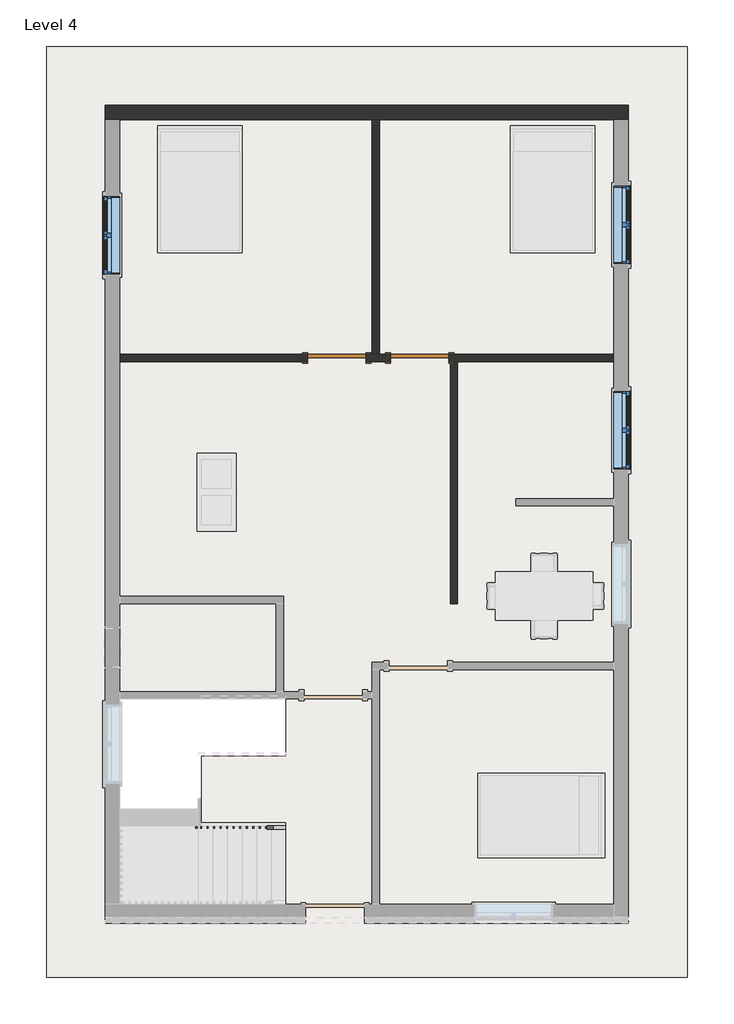
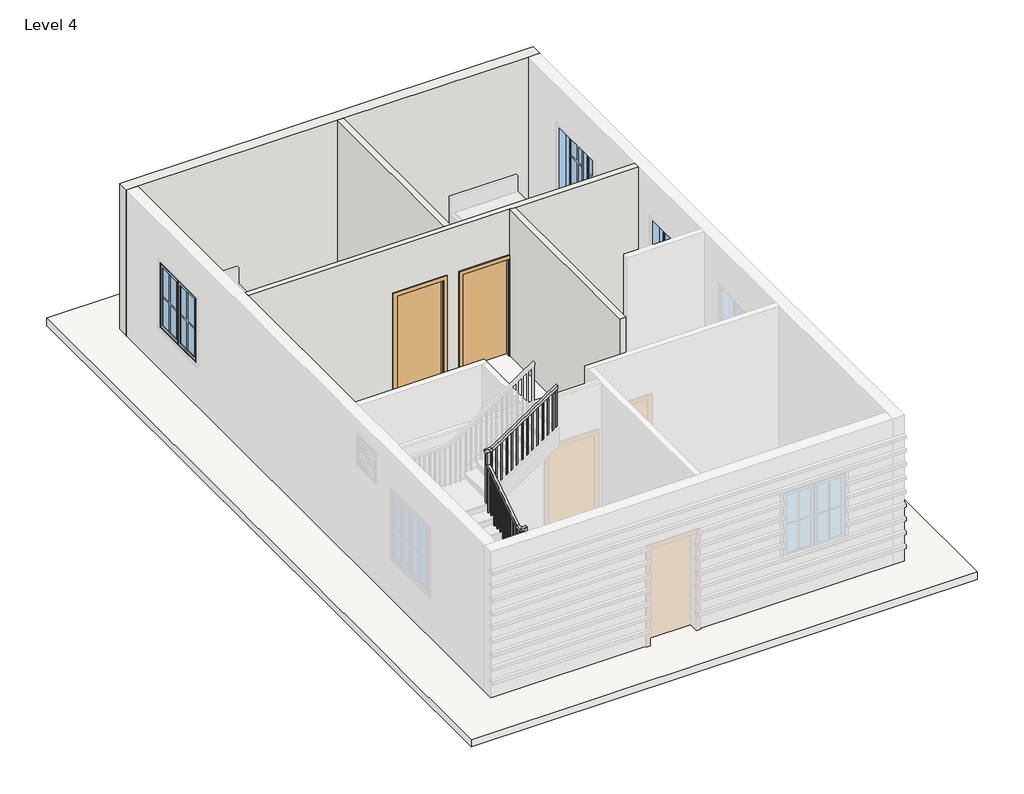
# One storey, part 2 of 3: 4 walls, 3 windows, 2 doors, 1 railing, 1 roof.
"""IFC4 building model written with IfcOpenShell, lengths in millimetres."""

from ifc_helpers import new_model, si_unit, frame, origin, place, context, project, spatial, polyline, outline, extrude, faceted_brep, transform, mapped, element, save
from components import single_flush_door_3_17d80c48, single_flush_door_3_5e62189b, window_casement_double_window_4_576b2d2c

model = new_model("IFC4")

# Units and contexts
model_context = context("Model", 3, world=origin())
ifc_project = project(units=[si_unit("LENGTHUNIT", "METRE", prefix="MILLI")], contexts=[model_context])

# Site, building, storey
site = spatial("IfcSite", under=ifc_project)
building = spatial("IfcBuilding", under=site)
storey = spatial("IfcBuildingStorey", under=building, Name="Level 4", Elevation=9448.8)

# Doors
placement = place(None, origin())
single_flush_door_3_shape = single_flush_door_3_17d80c48(model_context)
element("IfcDoor", 1, ObjectType="Single-Flush : DOOR 3'", at=placement, inside=storey, context=model_context, shape_type="MappedRepresentation", body=[
    mapped(single_flush_door_3_shape, transform((-1721.4617403, 2133.1073441, 9448.8), x_axis=(1.0, 0.0, 0.0), y_axis=(0.0, 1.0, 0.0), z_axis=(0.0, 0.0, 1.0))),
])
single_flush_door_3_2_shape = single_flush_door_3_5e62189b(model_context)
element("IfcDoor", 2, ObjectType="Single-Flush : DOOR 3'", at=placement, inside=storey, context=model_context, shape_type="MappedRepresentation", body=[
    mapped(single_flush_door_3_2_shape, transform((-426.0617403, 2133.1073441, 9448.8), x_axis=(-1.0, 0.0, 0.0), y_axis=(0.0, -1.0, 0.0), z_axis=(0.0, 0.0, 1.0))),
])

# Railing
element("IfcRailing", 3, ObjectType="Handrail - Rectangular", at=placement, inside=storey, context=model_context, shape_type="SolidModel", body=[
    faceted_brep([(-2515.2117403, -5213.8426559, 10515.6), (-2515.2117403, -5213.8426559, 10454.5459984), (-2515.2117403, -5163.0426559, 10454.5459984), (-2515.2117403, -5163.0426559, 10515.6), (-3810.6117403, -5213.8426559, 11379.2), (-3861.4117403, -5213.8426559, 11352.0126651), (-3861.4117403, -5163.0426559, 11352.0126651), (-3810.6117403, -5163.0426559, 11379.2), (-3810.6117403, -5213.8426559, 11633.2), (-3861.4117403, -5213.8426559, 11582.4), (-3861.4117403, -5163.0426559, 11582.4), (-3810.6117403, -5163.0426559, 11633.2), (-3937.6117403, -5213.8426559, 11633.2), (-3937.6117403, -5213.8426559, 11582.4), (-3886.8117403, -5163.0426559, 11582.4), (-3886.8117403, -5163.0426559, 11633.2), (-3937.6117403, -5086.8426559, 11633.2), (-3937.6117403, -5071.4616535, 11582.4), (-3886.8117403, -5071.4616535, 11582.4), (-3886.8117403, -5086.8426559, 11633.2), (-3937.6117403, -4096.2426559, 12293.6), (-3937.6117403, -4045.4426559, 12266.4126651), (-3886.8117403, -4045.4426559, 12266.4126651), (-3886.8117403, -4096.2426559, 12293.6), (-3937.6117403, -4096.2426559, 12547.6), (-3937.6117403, -4045.4426559, 12496.8), (-3886.8117403, -4045.4426559, 12496.8), (-3886.8117403, -4096.2426559, 12547.6), (-3937.6117403, -3969.2426559, 12547.6), (-3937.6117403, -3969.2426559, 12496.8), (-3886.8117403, -4020.0426559, 12496.8), (-3886.8117403, -4020.0426559, 12547.6), (-3810.6117403, -3969.2426559, 12547.6), (-3795.2307379, -3969.2426559, 12496.8), (-3795.2307379, -4020.0426559, 12496.8), (-3810.6117403, -4020.0426559, 12547.6), (-2515.2117403, -3969.2426559, 13411.2), (-2515.2117403, -4020.0426559, 13411.2), (-2515.2117403, -4020.0426559, 13350.1459984), (-2515.2117403, -3969.2426559, 13350.1459984)], [[[0, 1, 2, 3]], [[1, 0, 4, 5]], [[2, 1, 5, 6]], [[3, 2, 6, 7]], [[0, 3, 7, 4]], [[5, 4, 8, 9]], [[6, 5, 9, 10]], [[7, 6, 10, 11]], [[4, 7, 11, 8]], [[9, 8, 12, 13]], [[10, 9, 13, 14]], [[11, 10, 14, 15]], [[8, 11, 15, 12]], [[13, 12, 16, 17]], [[14, 13, 17, 18]], [[15, 14, 18, 19]], [[12, 15, 19, 16]], [[17, 16, 20, 21]], [[18, 17, 21, 22]], [[19, 18, 22, 23]], [[16, 19, 23, 20]], [[21, 20, 24, 25]], [[22, 21, 25, 26]], [[23, 22, 26, 27]], [[20, 23, 27, 24]], [[25, 24, 28, 29]], [[26, 25, 29, 30]], [[27, 26, 30, 31]], [[24, 27, 31, 28]], [[29, 28, 32, 33]], [[30, 29, 33, 34]], [[31, 30, 34, 35]], [[28, 31, 35, 32]], [[36, 37, 38, 39]], [[33, 32, 36, 39]], [[34, 33, 39, 38]], [[35, 34, 38, 37]], [[32, 35, 37, 36]]]),
    extrude(outline(polyline([(13305.6959984, -2581.8867403), (13292.9959984, -2600.9367403), (12344.4, -2600.9367403), (12344.4, -2581.8867403), (13305.6959984, -2581.8867403)])), frame((0.0, -4004.1676559, 0.0), z_axis=(0.0, 1.0, 0.0), x_axis=(0.0, 0.0, 1.0)), (0.0, 0.0, 1.0), 19.05),
    extrude(outline(polyline([(13237.9626651, -2683.4867403), (13225.2626651, -2702.5367403), (12344.4, -2702.5367403), (12344.4, -2683.4867403), (13237.9626651, -2683.4867403)])), frame((0.0, -4004.1676559, 0.0), z_axis=(0.0, 1.0, 0.0), x_axis=(0.0, 0.0, 1.0)), (0.0, 0.0, 1.0), 19.05),
    extrude(outline(polyline([(13170.2293317, -2785.0867403), (13157.5293317, -2804.1367403), (12192.0, -2804.1367403), (12192.0, -2785.0867403), (13170.2293317, -2785.0867403)])), frame((0.0, -4004.1676559, 0.0), z_axis=(0.0, 1.0, 0.0), x_axis=(0.0, 0.0, 1.0)), (0.0, 0.0, 1.0), 19.05),
    extrude(outline(polyline([(13102.4959984, -2886.6867403), (13089.7959984, -2905.7367403), (12192.0, -2905.7367403), (12192.0, -2886.6867403), (13102.4959984, -2886.6867403)])), frame((0.0, -4004.1676559, 0.0), z_axis=(0.0, 1.0, 0.0), x_axis=(0.0, 0.0, 1.0)), (0.0, 0.0, 1.0), 19.05),
    extrude(outline(polyline([(13034.7626651, -2988.2867403), (13022.0626651, -3007.3367403), (12039.6, -3007.3367403), (12039.6, -2988.2867403), (13034.7626651, -2988.2867403)])), frame((0.0, -4004.1676559, 0.0), z_axis=(0.0, 1.0, 0.0), x_axis=(0.0, 0.0, 1.0)), (0.0, 0.0, 1.0), 19.05),
    extrude(outline(polyline([(12967.0293317, -3089.8867403), (12954.3293317, -3108.9367403), (12039.6, -3108.9367403), (12039.6, -3089.8867403), (12967.0293317, -3089.8867403)])), frame((0.0, -4004.1676559, 0.0), z_axis=(0.0, 1.0, 0.0), x_axis=(0.0, 0.0, 1.0)), (0.0, 0.0, 1.0), 19.05),
    extrude(outline(polyline([(12899.2959984, -3191.4867403), (12886.5959984, -3210.5367403), (12039.6, -3210.5367403), (12039.6, -3191.4867403), (12899.2959984, -3191.4867403)])), frame((0.0, -4004.1676559, 0.0), z_axis=(0.0, 1.0, 0.0), x_axis=(0.0, 0.0, 1.0)), (0.0, 0.0, 1.0), 19.05),
    extrude(outline(polyline([(12831.5626651, -3293.0867403), (12818.8626651, -3312.1367403), (11887.2, -3312.1367403), (11887.2, -3293.0867403), (12831.5626651, -3293.0867403)])), frame((0.0, -4004.1676559, 0.0), z_axis=(0.0, 1.0, 0.0), x_axis=(0.0, 0.0, 1.0)), (0.0, 0.0, 1.0), 19.05),
    extrude(outline(polyline([(12763.8293317, -3394.6867403), (12751.1293317, -3413.7367403), (11887.2, -3413.7367403), (11887.2, -3394.6867403), (12763.8293317, -3394.6867403)])), frame((0.0, -4004.1676559, 0.0), z_axis=(0.0, 1.0, 0.0), x_axis=(0.0, 0.0, 1.0)), (0.0, 0.0, 1.0), 19.05),
    extrude(outline(polyline([(12696.0959984, -3496.2867403), (12683.3959984, -3515.3367403), (11734.8, -3515.3367403), (11734.8, -3496.2867403), (12696.0959984, -3496.2867403)])), frame((0.0, -4004.1676559, 0.0), z_axis=(0.0, 1.0, 0.0), x_axis=(0.0, 0.0, 1.0)), (0.0, 0.0, 1.0), 19.05),
    extrude(outline(polyline([(12628.3626651, -3597.8867403), (12615.6626651, -3616.9367403), (11734.8, -3616.9367403), (11734.8, -3597.8867403), (12628.3626651, -3597.8867403)])), frame((0.0, -4004.1676559, 0.0), z_axis=(0.0, 1.0, 0.0), x_axis=(0.0, 0.0, 1.0)), (0.0, 0.0, 1.0), 19.05),
    extrude(outline(polyline([(12560.6293317, -3699.4867403), (12547.9293317, -3718.5367403), (11582.4, -3718.5367403), (11582.4, -3699.4867403), (12560.6293317, -3699.4867403)])), frame((0.0, -4004.1676559, 0.0), z_axis=(0.0, 1.0, 0.0), x_axis=(0.0, 0.0, 1.0)), (0.0, 0.0, 1.0), 19.05),
    extrude(outline(polyline([(12492.8959984, -3801.0867403), (12480.1959984, -3820.1367403), (11582.4, -3820.1367403), (11582.4, -3801.0867403), (12492.8959984, -3801.0867403)])), frame((0.0, -4004.1676559, 0.0), z_axis=(0.0, 1.0, 0.0), x_axis=(0.0, 0.0, 1.0)), (0.0, 0.0, 1.0), 19.05),
    extrude(outline(polyline([(-3902.6867403, -4080.3676559), (-3921.7367403, -4080.3676559), (-3921.7367403, -4061.3176559), (-3902.6867403, -4061.3176559), (-3902.6867403, -4080.3676559)])), frame((0.0, 0.0, 11277.6), z_axis=(0.0, 0.0, 1.0), x_axis=(1.0, 0.0, 0.0)), (0.0, 0.0, 1.0), 1219.2),
    extrude(outline(polyline([(-4181.9676559, 12175.3959984), (-4162.9176559, 12188.0959984), (-4162.9176559, 11277.6), (-4181.9676559, 11277.6), (-4181.9676559, 12175.3959984)])), frame((-3921.7367403, 0.0, 0.0), z_axis=(1.0, 0.0, 0.0), x_axis=(0.0, 1.0, 0.0)), (0.0, 0.0, 1.0), 19.05),
    extrude(outline(polyline([(-4283.5676559, 12107.6626651), (-4264.5176559, 12120.3626651), (-4264.5176559, 11125.2), (-4283.5676559, 11125.2), (-4283.5676559, 12107.6626651)])), frame((-3921.7367403, 0.0, 0.0), z_axis=(1.0, 0.0, 0.0), x_axis=(0.0, 1.0, 0.0)), (0.0, 0.0, 1.0), 19.05),
    extrude(outline(polyline([(-4385.1676559, 12039.9293317), (-4366.1176559, 12052.6293317), (-4366.1176559, 11125.2), (-4385.1676559, 11125.2), (-4385.1676559, 12039.9293317)])), frame((-3921.7367403, 0.0, 0.0), z_axis=(1.0, 0.0, 0.0), x_axis=(0.0, 1.0, 0.0)), (0.0, 0.0, 1.0), 19.05),
    extrude(outline(polyline([(-4486.7676559, 11972.1959984), (-4467.7176559, 11984.8959984), (-4467.7176559, 11125.2), (-4486.7676559, 11125.2), (-4486.7676559, 11972.1959984)])), frame((-3921.7367403, 0.0, 0.0), z_axis=(1.0, 0.0, 0.0), x_axis=(0.0, 1.0, 0.0)), (0.0, 0.0, 1.0), 19.05),
    extrude(outline(polyline([(-4588.3676559, 11904.4626651), (-4569.3176559, 11917.1626651), (-4569.3176559, 10972.8), (-4588.3676559, 10972.8), (-4588.3676559, 11904.4626651)])), frame((-3921.7367403, 0.0, 0.0), z_axis=(1.0, 0.0, 0.0), x_axis=(0.0, 1.0, 0.0)), (0.0, 0.0, 1.0), 19.05),
    extrude(outline(polyline([(-4689.9676559, 11836.7293317), (-4670.9176559, 11849.4293317), (-4670.9176559, 10972.8), (-4689.9676559, 10972.8), (-4689.9676559, 11836.7293317)])), frame((-3921.7367403, 0.0, 0.0), z_axis=(1.0, 0.0, 0.0), x_axis=(0.0, 1.0, 0.0)), (0.0, 0.0, 1.0), 19.05),
    extrude(outline(polyline([(-4791.5676559, 11768.9959984), (-4772.5176559, 11781.6959984), (-4772.5176559, 10820.4), (-4791.5676559, 10820.4), (-4791.5676559, 11768.9959984)])), frame((-3921.7367403, 0.0, 0.0), z_axis=(1.0, 0.0, 0.0), x_axis=(0.0, 1.0, 0.0)), (0.0, 0.0, 1.0), 19.05),
    extrude(outline(polyline([(-4893.1676559, 11701.2626651), (-4874.1176559, 11713.9626651), (-4874.1176559, 10820.4), (-4893.1676559, 10820.4), (-4893.1676559, 11701.2626651)])), frame((-3921.7367403, 0.0, 0.0), z_axis=(1.0, 0.0, 0.0), x_axis=(0.0, 1.0, 0.0)), (0.0, 0.0, 1.0), 19.05),
    extrude(outline(polyline([(-4994.7676559, 11633.5293317), (-4975.7176559, 11646.2293317), (-4975.7176559, 10668.0), (-4994.7676559, 10668.0), (-4994.7676559, 11633.5293317)])), frame((-3921.7367403, 0.0, 0.0), z_axis=(1.0, 0.0, 0.0), x_axis=(0.0, 1.0, 0.0)), (0.0, 0.0, 1.0), 19.05),
    extrude(outline(polyline([(-5096.3676559, 11565.7959984), (-5077.3176559, 11578.4959984), (-5077.3176559, 10668.0), (-5096.3676559, 10668.0), (-5096.3676559, 11565.7959984)])), frame((-3921.7367403, 0.0, 0.0), z_axis=(1.0, 0.0, 0.0), x_axis=(0.0, 1.0, 0.0)), (0.0, 0.0, 1.0), 19.05),
    extrude(outline(polyline([(-3826.4867403, -5178.9176559), (-3826.4867403, -5197.9676559), (-3845.5367403, -5197.9676559), (-3845.5367403, -5178.9176559), (-3826.4867403, -5178.9176559)])), frame((0.0, 0.0, 10363.2), z_axis=(0.0, 0.0, 1.0), x_axis=(1.0, 0.0, 0.0)), (0.0, 0.0, 1.0), 1219.2),
    extrude(outline(polyline([(11260.9959984, -3724.8867403), (11273.6959984, -3743.9367403), (10363.2, -3743.9367403), (10363.2, -3724.8867403), (11260.9959984, -3724.8867403)])), frame((0.0, -5197.9676559, 0.0), z_axis=(0.0, 1.0, 0.0), x_axis=(0.0, 0.0, 1.0)), (0.0, 0.0, 1.0), 19.05),
    extrude(outline(polyline([(11193.2626651, -3623.2867403), (11205.9626651, -3642.3367403), (10210.8, -3642.3367403), (10210.8, -3623.2867403), (11193.2626651, -3623.2867403)])), frame((0.0, -5197.9676559, 0.0), z_axis=(0.0, 1.0, 0.0), x_axis=(0.0, 0.0, 1.0)), (0.0, 0.0, 1.0), 19.05),
    extrude(outline(polyline([(11125.5293317, -3521.6867403), (11138.2293317, -3540.7367403), (10210.8, -3540.7367403), (10210.8, -3521.6867403), (11125.5293317, -3521.6867403)])), frame((0.0, -5197.9676559, 0.0), z_axis=(0.0, 1.0, 0.0), x_axis=(0.0, 0.0, 1.0)), (0.0, 0.0, 1.0), 19.05),
    extrude(outline(polyline([(11057.7959984, -3420.0867403), (11070.4959984, -3439.1367403), (10210.8, -3439.1367403), (10210.8, -3420.0867403), (11057.7959984, -3420.0867403)])), frame((0.0, -5197.9676559, 0.0), z_axis=(0.0, 1.0, 0.0), x_axis=(0.0, 0.0, 1.0)), (0.0, 0.0, 1.0), 19.05),
    extrude(outline(polyline([(10990.0626651, -3318.4867403), (11002.7626651, -3337.5367403), (10058.4, -3337.5367403), (10058.4, -3318.4867403), (10990.0626651, -3318.4867403)])), frame((0.0, -5197.9676559, 0.0), z_axis=(0.0, 1.0, 0.0), x_axis=(0.0, 0.0, 1.0)), (0.0, 0.0, 1.0), 19.05),
    extrude(outline(polyline([(10922.3293317, -3216.8867403), (10935.0293317, -3235.9367403), (10058.4, -3235.9367403), (10058.4, -3216.8867403), (10922.3293317, -3216.8867403)])), frame((0.0, -5197.9676559, 0.0), z_axis=(0.0, 1.0, 0.0), x_axis=(0.0, 0.0, 1.0)), (0.0, 0.0, 1.0), 19.05),
    extrude(outline(polyline([(10854.5959984, -3115.2867403), (10867.2959984, -3134.3367403), (9906.0, -3134.3367403), (9906.0, -3115.2867403), (10854.5959984, -3115.2867403)])), frame((0.0, -5197.9676559, 0.0), z_axis=(0.0, 1.0, 0.0), x_axis=(0.0, 0.0, 1.0)), (0.0, 0.0, 1.0), 19.05),
    extrude(outline(polyline([(10786.8626651, -3013.6867403), (10799.5626651, -3032.7367403), (9906.0, -3032.7367403), (9906.0, -3013.6867403), (10786.8626651, -3013.6867403)])), frame((0.0, -5197.9676559, 0.0), z_axis=(0.0, 1.0, 0.0), x_axis=(0.0, 0.0, 1.0)), (0.0, 0.0, 1.0), 19.05),
    extrude(outline(polyline([(10719.1293317, -2912.0867403), (10731.8293317, -2931.1367403), (9753.6, -2931.1367403), (9753.6, -2912.0867403), (10719.1293317, -2912.0867403)])), frame((0.0, -5197.9676559, 0.0), z_axis=(0.0, 1.0, 0.0), x_axis=(0.0, 0.0, 1.0)), (0.0, 0.0, 1.0), 19.05),
    extrude(outline(polyline([(10651.3959984, -2810.4867403), (10664.0959984, -2829.5367403), (9753.6, -2829.5367403), (9753.6, -2810.4867403), (10651.3959984, -2810.4867403)])), frame((0.0, -5197.9676559, 0.0), z_axis=(0.0, 1.0, 0.0), x_axis=(0.0, 0.0, 1.0)), (0.0, 0.0, 1.0), 19.05),
    extrude(outline(polyline([(10583.6626651, -2708.8867403), (10596.3626651, -2727.9367403), (9601.2, -2727.9367403), (9601.2, -2708.8867403), (10583.6626651, -2708.8867403)])), frame((0.0, -5197.9676559, 0.0), z_axis=(0.0, 1.0, 0.0), x_axis=(0.0, 0.0, 1.0)), (0.0, 0.0, 1.0), 19.05),
    extrude(outline(polyline([(10515.9293317, -2607.2867403), (10528.6293317, -2626.3367403), (9601.2, -2626.3367403), (9601.2, -2607.2867403), (10515.9293317, -2607.2867403)])), frame((0.0, -5197.9676559, 0.0), z_axis=(0.0, 1.0, 0.0), x_axis=(0.0, 0.0, 1.0)), (0.0, 0.0, 1.0), 19.05),
    extrude(outline(polyline([(-3902.6867403, -4004.1676559), (-3921.7367403, -4004.1676559), (-3921.7367403, -3985.1176559), (-3902.6867403, -3985.1176559), (-3902.6867403, -4004.1676559)])), frame((0.0, 0.0, 11430.0), z_axis=(0.0, 0.0, 1.0), x_axis=(1.0, 0.0, 0.0)), (0.0, 0.0, 1.0), 1066.8),
    extrude(outline(polyline([(-3902.6867403, -5178.9176559), (-3902.6867403, -5197.9676559), (-3921.7367403, -5197.9676559), (-3921.7367403, -5178.9176559), (-3902.6867403, -5178.9176559)])), frame((0.0, 0.0, 10515.6), z_axis=(0.0, 0.0, 1.0), x_axis=(1.0, 0.0, 0.0)), (0.0, 0.0, 1.0), 1066.8),
    extrude(outline(polyline([(13350.1459984, -2515.2117403), (13337.4459984, -2534.2617403), (12344.4, -2534.2617403), (12344.4, -2515.2117403), (13350.1459984, -2515.2117403)])), frame((0.0, -4004.1676559, 0.0), z_axis=(0.0, 1.0, 0.0), x_axis=(0.0, 0.0, 1.0)), (0.0, 0.0, 1.0), 19.05),
    extrude(outline(polyline([(10454.5459984, -2515.2117403), (10467.2459984, -2534.2617403), (9601.2, -2534.2617403), (9601.2, -2515.2117403), (10454.5459984, -2515.2117403)])), frame((0.0, -5197.9676559, 0.0), z_axis=(0.0, 1.0, 0.0), x_axis=(0.0, 0.0, 1.0)), (0.0, 0.0, 1.0), 19.05),
])

# Roof
element("IfcRoof", 4, ObjectType="ROOF 6\"", at=placement, inside=storey, context=model_context, shape_type="SweptSolid", body=[
    extrude(outline(polyline([(-6249.0117403, -7525.2426559), (-6249.0117403, 6990.8573441), (3745.8882597, 6990.8573441), (3745.8882597, -7525.2426559), (-6249.0117403, -7525.2426559)]), holes=[polyline([(-5156.8117403, -3131.0426559), (-5156.8117403, -6433.0426559), (-2515.2117403, -6433.0426559), (-2515.2117403, -5112.2426559), (-3836.0117403, -5112.2426559), (-3836.0117403, -4070.8426559), (-2515.2117403, -4070.8426559), (-2515.2117403, -3131.0426559), (-5156.8117403, -3131.0426559)])]), frame((0.0, 0.0, 9296.4), z_axis=(0.0, 0.0, 1.0), x_axis=(1.0, 0.0, 0.0)), (0.0, 0.0, 1.0), 152.4),
])

# Walls
element("IfcWall", 5, ObjectType="ALL 4.5\"", at=placement, inside=storey, context=model_context, shape_type="Brep", body=[
    faceted_brep([(-1264.2617403, 2075.9573441, 9448.8), (-883.2617403, 2075.9573441, 9448.8), (-883.2617403, 2075.9573441, 11480.8), (31.1382597, 2075.9573441, 11480.8), (31.1382597, 2075.9573441, 9448.8), (50.1882597, 2075.9573441, 9448.8), (164.4882597, 2075.9573441, 9448.8), (2602.8882597, 2075.9573441, 9448.8), (2602.8882597, 2075.9573441, 12496.8), (164.4882597, 2075.9573441, 12496.8), (50.1882597, 2075.9573441, 12496.8), (-5106.0117403, 2075.9573441, 12496.8), (-5106.0117403, 2075.9573441, 9448.8), (-2178.6617403, 2075.9573441, 9448.8), (-2178.6617403, 2075.9573441, 11480.8), (-1264.2617403, 2075.9573441, 11480.8), (-883.2617403, 2190.2573441, 11480.8), (-883.2617403, 2190.2573441, 9448.8), (-1054.7117403, 2190.2573441, 9448.8), (-1169.0117403, 2190.2573441, 9448.8), (-1264.2617403, 2190.2573441, 9448.8), (-1264.2617403, 2190.2573441, 11480.8), (-2178.6617403, 2190.2573441, 11480.8), (-2178.6617403, 2190.2573441, 9448.8), (-5106.0117403, 2190.2573441, 9448.8), (-5106.0117403, 2190.2573441, 12496.8), (-1169.0117403, 2190.2573441, 12496.8), (-1054.7117403, 2190.2573441, 12496.8), (2602.8882597, 2190.2573441, 12496.8), (2602.8882597, 2190.2573441, 9448.8), (31.1382597, 2190.2573441, 9448.8), (31.1382597, 2190.2573441, 11480.8)], [[[0, 1, 2, 3, 4, 5, 6, 7, 8, 9, 10, 11, 12, 13, 14, 15]], [[16, 17, 18, 19, 20, 21, 22, 23, 24, 25, 26, 27, 28, 29, 30, 31]], [[13, 12, 24, 23]], [[30, 29, 7, 6, 5, 4]], [[20, 19, 18, 17, 1, 0]], [[8, 7, 29, 28]], [[12, 11, 25, 24]], [[21, 20, 0, 15]], [[22, 21, 15, 14]], [[23, 22, 14, 13]], [[2, 1, 17, 16]], [[3, 2, 16, 31]], [[4, 3, 31, 30]], [[11, 10, 9, 8, 28, 27, 26, 25]]]),
])
element("IfcWall", 6, ObjectType="ALL 4.5\"", at=placement, inside=storey, context=model_context, shape_type="SweptSolid", body=[
    extrude(outline(polyline([(50.1882597, -1695.9426559), (50.1882597, 2075.9573441), (164.4882597, 2075.9573441), (164.4882597, -1695.9426559), (50.1882597, -1695.9426559)])), frame((0.0, 0.0, 9448.8), z_axis=(0.0, 0.0, 1.0), x_axis=(1.0, 0.0, 0.0)), (0.0, 0.0, 1.0), 3048.0),
])
element("IfcWall", 7, ObjectType="ALL 4.5\"", at=placement, inside=storey, context=model_context, shape_type="SweptSolid", body=[
    extrude(outline(polyline([(-1169.0117403, 2190.2573441), (-1169.0117403, 5847.8573441), (-1054.7117403, 5847.8573441), (-1054.7117403, 2190.2573441), (-1169.0117403, 2190.2573441)])), frame((0.0, 0.0, 9448.8), z_axis=(0.0, 0.0, 1.0), x_axis=(1.0, 0.0, 0.0)), (0.0, 0.0, 1.0), 3048.0),
])
element("IfcWall", 8, ObjectType="WALL 9\"", at=placement, inside=storey, context=model_context, shape_type="Brep", body=[
    faceted_brep([(-5334.6117403, 5847.8573441, 9448.8), (-5106.0117403, 5847.8573441, 9448.8), (-1169.0117403, 5847.8573441, 9448.8), (-1054.7117403, 5847.8573441, 9448.8), (2602.8882597, 5847.8573441, 9448.8), (2831.4882597, 5847.8573441, 9448.8), (2831.4882597, 5847.8573441, 12496.8), (2602.8882597, 5847.8573441, 12496.8), (-1054.7117403, 5847.8573441, 12496.8), (-1169.0117403, 5847.8573441, 12496.8), (-5106.0117403, 5847.8573441, 12496.8), (-5334.6117403, 5847.8573441, 12496.8), (-5334.6117403, 6076.4573441, 9448.8), (-5334.6117403, 6076.4573441, 12496.8), (2831.4882597, 6076.4573441, 12496.8), (2831.4882597, 6076.4573441, 9448.8)], [[[0, 1, 2, 3, 4, 5, 6, 7, 8, 9, 10, 11]], [[12, 13, 14, 15]], [[5, 4, 3, 2, 1, 0, 12, 15]], [[6, 5, 15, 14]], [[0, 11, 13, 12]], [[11, 10, 9, 8, 7, 6, 14, 13]]]),
])

# Windows
window_casement_double_window_4_shape = window_casement_double_window_4_576b2d2c(model_context)
element("IfcWindow", 9, ObjectType="Window-Casement-Double : WINDOW 4'", at=placement, inside=storey, context=model_context, shape_type="MappedRepresentation", body=[
    mapped(window_casement_double_window_4_shape, transform((-5220.3117403, 4047.6323441, 9448.8), x_axis=(0.0, 1.0, 0.0), y_axis=(-1.0, 0.0, 0.0), z_axis=(0.0, 0.0, 1.0))),
])
element("IfcWindow", 10, ObjectType="Window-Casement-Double : WINDOW 4'", at=placement, inside=storey, context=model_context, shape_type="MappedRepresentation", body=[
    mapped(window_casement_double_window_4_shape, transform((2717.1882597, 4209.5573441, 9448.8), x_axis=(0.0, -1.0, 0.0), y_axis=(1.0, 0.0, 0.0), z_axis=(0.0, 0.0, 1.0))),
])
element("IfcWindow", 11, ObjectType="Window-Casement-Double : WINDOW 4'", at=placement, inside=storey, context=model_context, shape_type="MappedRepresentation", body=[
    mapped(window_casement_double_window_4_shape, transform((2717.1882597, 1009.1573441, 9448.8), x_axis=(0.0, -1.0, 0.0), y_axis=(1.0, 0.0, 0.0), z_axis=(0.0, 0.0, 1.0))),
])

save(model, "model.ifc")

# Revit data of these elements
# Type "Single-Flush : DOOR 3'"
#   Type Mark = "8"
#   Construction Type Id = "MDOOR"
#   Assembly Code = "C1020"
#   Analytic Construction = "Metal"
#   Thickness = 0' - 2"
#   Heat Transfer Coefficient (U) = 0.651978 BTU/(h·ft²·°F)
#   Height = 6' - 8"
#   Trim Projection Ext = 0' - 1"
#   Trim Projection Int = 0' - 1"
#   Trim Width = 0' - 3"
#   Width = 3' - 0"
#   Define Thermal Properties by = 1
#   Door Material = Door - Panel
#   Frame Material = Door - Frame
#   Visual Light Transmittance = 0
#   Solar Heat Gain Coefficient = 0
#   Function = (empty or 0)
#   Wall Closure = (empty or 0)
# Type "Handrail - Rectangular"
#   Assembly Code = "C2010400"
#   built-in parameter 1008612 = 0.0416667 (stored number, unit not read)
#   built-in parameter 1008611 = 0.0416667 (stored number, unit not read)
#   built-in parameter 1008609 = 0.333333 (stored number, unit not read)
#   built-in parameter 1008604 = 0.166667 (stored number, unit not read)
#   built-in parameter 1008603 = 0.166667 (stored number, unit not read)
#   Railing Height = 3' - 0"
#   built-in parameter 1008630 = 2
#   built-in parameter 1008610 = 2
#   built-in parameter 1008618 = Baluster - Square : 3/4"
# Type "ROOF 6\""
#   Assembly Code = "B1020"
#   Layers, outside or top first: 0' - 6" no material (function 1)
# Type "ALL 4.5\""
#   Assembly Code = "B2010"
#   Layers, outside or top first: 0' - 4 1/2" no material (function 1)
# Type "WALL 9\""
#   Assembly Code = "B2010"
#   Layers, outside or top first: 0' - 9" "Carpet (1)" (function 1)
# Type "Window-Casement-Double : WINDOW 4'"
#   Type Mark = "18"
#   Fire Rating = "0.5h"
#   Assembly Code = "B2020100"
#   Analytic Construction = "Double glazing - domestic"
#   Frame Extension [instance default] = 0' - 0 1/4"
#   Window Inset [instance default] = 0' - 0"
#   Wall Thickness [instance default] = 0' - 6"
#   Interior Wall Closure [instance default] = 0' - 2 1/4"
#   Half Width = 2' - 0"
#   Visual Light Transmittance = 0.81
#   Thermal Resistance (R) = 1.8146 (h·ft²·°F)/BTU
#   Solar Heat Gain Coefficient = 0.76
#   Rough Width = 4' - 0 1/2"
#   Rough Height = 4' - 5 1/2"
#   Height = 4' - 5"
#   Heat Transfer Coefficient (U) = 0.5511 BTU/(h·ft²·°F)
#   Exterior Wall Closure [instance default] = 0' - 1 1/4"
#   Extension Jamb [instance default] = 0' - 2 1/4"
#   Default Sill Height = 3' - 0"
#   Width = 4' - 0"
#   Muntin Visibility = yes
#   Interior Trim Visibility [instance default] = yes
#   Exterior Trim Visibility [instance default] = yes
#   Extension Jamb Visibility [instance default] = yes
#   Interior Trim Material = Wood - Stained
#   Muntin Pattern = Muntin Pattern_2x2 : Muntin Pattern_2x2
#   Interior Trim = Trim-Window-Interior-Flat : Picture Frame
#   Interior Frame Material = Wood - Stained
#   Glass Panel Material = Glass
#   Exterior Trim Material = Clad - White
#   Exterior Trim = Trim-Window-Exterior-Flat : with Sill
#   Exterior Frame Material = Clad - White
#   Wall Closure = (empty or 0)
# Elements 1, 2 (IfcDoor, "Single-Flush : DOOR 3'")
#   Phase Created = New Construction
#   Materials on its faces: "Door - Frame", "Door - Panel"
# Element 3 (IfcRailing, "Handrail - Rectangular")
#   Phase Created = New Construction
#   Materials on its faces: "Clad - White"
# Element 4 (IfcRoof, "ROOF 6\"")
#   built-in parameter 1001705 = 31 (stored number, unit not read)
#   built-in parameter 1001701 = -0.5 (stored number, unit not read)
#   built-in parameter 1001710 = 33615
#   Phase Created = New Construction
#   Materials on its faces: "Clad - White", "Default Roof", "Softwood, Lumber"
# Elements 5, 6, 7 (IfcWall, "ALL 4.5\"")
#   Top Offset = 0' - 0"
#   Base Offset = 0' - 0"
#   Unconnected Height = 10' - 0"
#   wall height = 10' - 0"
#   Phase Created = New Construction
#   Base Constraint = Level 4
#   Materials on its faces: "Default Wall"
# Element 8 (IfcWall, "WALL 9\"")
#   Top Offset = 0' - 0"
#   Base Offset = 0' - 0"
#   Unconnected Height = 10' - 0"
#   wall height = 10' - 0"
#   Phase Created = New Construction
#   Base Constraint = Level 4
#   Materials on its faces: "Carpet (1)", "Wood - Stained"
# Element 9 (IfcWindow, "Window-Casement-Double : WINDOW 4'")
#   Mark = "23"
#   Window Inset = 0' - 0"
#   Interior Wall Closure = 0' - 2 1/4"
#   Frame Extension = 0' - 0 1/4"
#   Exterior Wall Closure = 0' - 1 1/4"
#   Interior Trim Visibility = yes
#   Exterior Trim Visibility = yes
#   Phase Created = New Construction
#   Materials on its faces: "Wood - Stained", "Glass", "Clad - White"
# Element 10 (IfcWindow, "Window-Casement-Double : WINDOW 4'")
#   Mark = "24"
#   Window Inset = 0' - 0"
#   Interior Wall Closure = 0' - 2 1/4"
#   Frame Extension = 0' - 0 1/4"
#   Exterior Wall Closure = 0' - 1 1/4"
#   Interior Trim Visibility = yes
#   Exterior Trim Visibility = yes
#   Phase Created = New Construction
#   Materials on its faces: "Wood - Stained", "Glass", "Clad - White"
# Element 11 (IfcWindow, "Window-Casement-Double : WINDOW 4'")
#   Mark = "25"
#   Window Inset = 0' - 0"
#   Interior Wall Closure = 0' - 2 1/4"
#   Frame Extension = 0' - 0 1/4"
#   Exterior Wall Closure = 0' - 1 1/4"
#   Interior Trim Visibility = yes
#   Exterior Trim Visibility = yes
#   Phase Created = New Construction
#   Materials on its faces: "Wood - Stained", "Glass", "Clad - White"
# Materials
#   "Door - Panel": class "Wood", colour RGB 210 159 95, transparency 0, Cost = 0
#   "Door - Frame": colour RGB 118 70 51, transparency 0, Cost = 0
#   "Carpet (1)": class "Carpet", colour RGB 124 80 67, transparency 0, Description = "Interior finish", Cost = 0
#   "Wood - Stained": class "Wood", colour RGB 224 178 126, transparency 0, Cost = 0
#   "Glass": class "Glass", colour RGB 0 128 192, transparency 0.75, Description = "Soda Lime Glass", Cost = 0
#   "Clad - White": class "Wood", colour RGB 242 242 238, transparency 0, Cost = 0
#   "Default Roof": colour RGB 88 101 114, transparency 0, Cost = 0
#   "Softwood, Lumber": class "Wood", colour RGB 223 192 134, transparency 0, Description = "Pinus Echinata", Cost = 0
#   "Default Wall": colour RGB 128 128 128, transparency 0, Cost = 0
